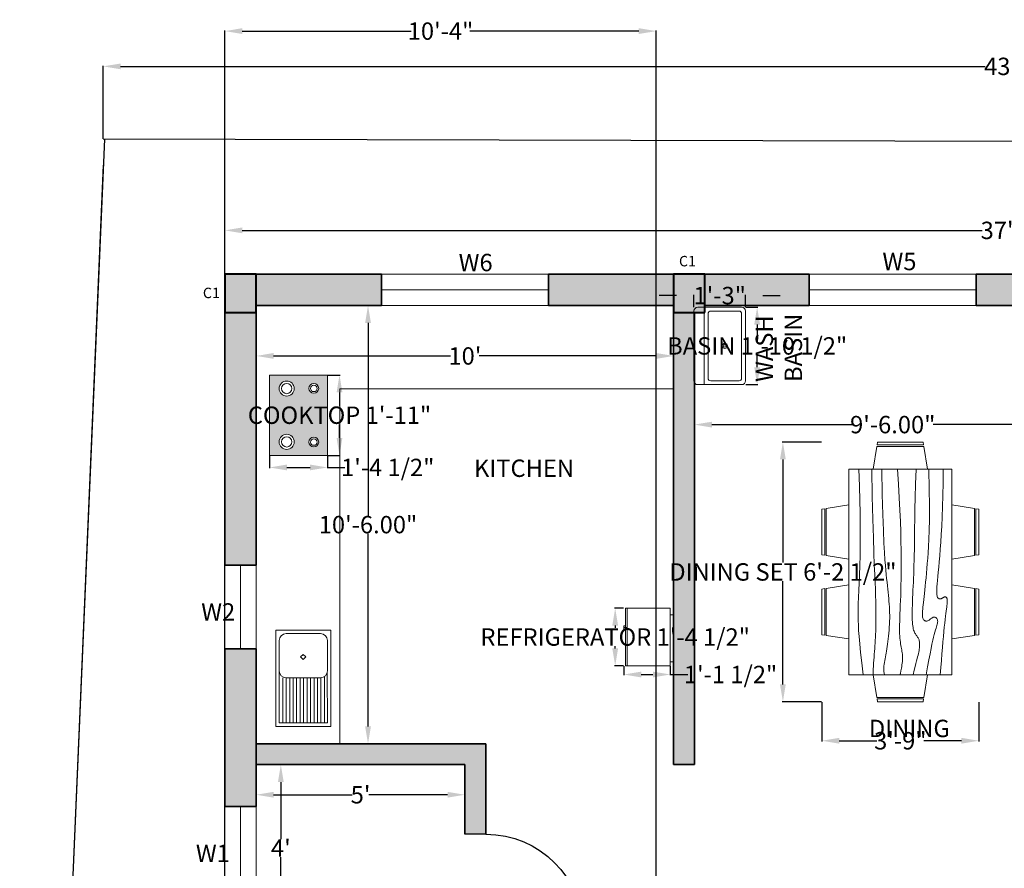
# Model space of a CAD drawing. Units: inches. Extents: x 23868 to 24454, y 31838 to 32477.
# Tile 3 of 4: x 23868 to 24151, y 32233 to 32477. Entities that reach past the tile are written whole.
import ezdxf

# ---------------------------------------------------------------- set-up
doc = ezdxf.new("R2010")
doc.units = ezdxf.units.IN
for name, color, linetype, lineweight in [('A-ANNO-DIMS', 2, 'Continuous', 18), ('A-AREA-IDEN', 7, 'Continuous', 25), ('A-COLS', 7, 'Continuous', 40), ('A-EQPM', 30, 'Continuous', 18), ('A-FIXT-PATT', 30, 'Continuous', 13), ('A-FLOR-CASE', 30, 'Continuous', 18), ('A-FLOR-FIXT', 30, 'Continuous', 18), ('A-FURN', 30, 'Continuous', 18), ('A-GLAZ', 5, 'Continuous', 18), ('A-WALL', 7, 'Continuous', 35), ('C-PROP', 7, 'Continuous', 25), ('door', 1, 'Continuous', 25), ('text', 7, 'Continuous', 18)]:
    doc.layers.add(name, color=color, linetype=linetype, lineweight=lineweight)
doc.layers.add('A-COLS-PATT', color=67, linetype='Continuous', lineweight=13, true_color=0x727430)
doc.layers.add('A-WALL-PATT', color=250, linetype='Continuous', lineweight=13, true_color=0x413a3c)
doc.styles.get("Standard").update_dxf_attribs({"font": 'arial.ttf', "height": 5})
doc.styles.add('style1', font='arial.ttf', dxfattribs={"height": 3})
doc.dimstyles.get("Standard").update_dxf_attribs({"dimtxt": 5, "dimasz": 5, "dimexe": 0.18, "dimexo": 0.0625, "dimgap": 0.09, "dimtad": 0, "dimtih": 1, "dimtoh": 1, "dimzin": 0, "dimdsep": 46, "dimlunit": 3, "dimtxsty": 'Standard', "dimcen": 0.09, "dimadec": 0, "dimazin": 0, "dimtfac": 1, "dimtofl": 0, "dimtmove": 0, "dimatfit": 3, "dimfxl": 1, "dimtolj": 1, "dimtzin": 0, "dimarcsym": 0})

# ---------------------------------------------------------------- blocks, each defined once
blk = doc.blocks.new('*U5')
for p, q in [((0, 0), (0, -6)), ((28, 0), (28, -6))]:
    blk.add_line(p, q)
blk.add_lwpolyline([(0, 0), (0, 28), (1.75, 28), (1.75, 0)], close=True)
blk.add_arc((0, 0), 28, 0, 90)
blk = doc.blocks.new('stov')
h = blk.add_hatch(color=256)
h.dxf.hatch_style = 1
h.set_gradient(color1=(255, 255, 255), color2=(147, 149, 152), name='CYLINDER')
h.paths.add_polyline_path([(0, 0), (16.67, 0), (16.67, 23.1), (0, 23.1)])
h.paths.add_polyline_path([(2.78, 19.21, -1), (7.12, 19.21, -1)], flags=16)
h.paths.add_polyline_path([(3.47, 19.21, -1), (6.43, 19.21, -1)], flags=0)
h.paths.add_polyline_path([(7.12, 3.89, -1), (2.78, 3.89, -1)], flags=16)
h.paths.add_polyline_path([(6.43, 3.89, -1), (3.47, 3.89, -1)], flags=0)
h.paths.add_polyline_path([(11.35, 19.27, -1), (14.15, 19.27, -1)], flags=16)
h.paths.add_polyline_path([(11.81, 19.27, -1), (13.68, 19.27, -1)], flags=0)
h.paths.add_polyline_path([(14.15, 3.83, -1), (11.35, 3.83, -1)], flags=16)
blk.add_lwpolyline([(16.67, 0), (0, 0), (0, 23.1), (16.67, 23.1)], close=True)
for centre, radius in [((4.95, 19.21), 2.17), ((4.95, 19.21), 2.17), ((4.95, 19.21), 1.48), ((12.75, 19.27), 1.4), ((12.75, 19.27), 0.936), ((4.95, 3.89), 2.17), ((4.95, 3.89), 2.17), ((4.95, 3.89), 1.48), ((12.75, 3.83), 1.4), ((12.75, 3.83), 0.936)]:
    blk.add_circle(centre, radius)
blk = doc.blocks.new('Refrigerator-2 door - 36 in top')
for p, q in [((0, -26.999999), (36, -26.999999)), ((11, -27.999999), (11, -28.999999)), ((11, -28.999999), (13, -28.999999)), ((12, -26.999999), (12, -28.999999)), ((13, -28.999999), (13, -27.999999))]:
    blk.add_line(p, q)
blk.add_lwpolyline([(0, -27.999999), (0, 0), (36, 0), (36, -27.999999)], close=True)
blk = doc.blocks.new('Sink-single - 30 in top')
blk.add_line((-15, -3.999996), (15, -3.999996))
for points in [[(-13.5, 0), (13.5, 0)], [(-15, -18.499996), (-15, -1.5)], [(15, -1.5), (15, -18.499996)], [(-13.5, -17.499996), (-13.5, -6.499996)], [(-12.5, -5.499996), (12.5, -5.499996)], [(13.5, -6.499996), (13.5, -17.499996)], [(12.5, -18.499996), (-12.5, -18.499996)], [(13.5, -19.999996), (-13.5, -19.999996)]]:
    blk.add_lwpolyline(points)
for radius in [1, 0.5]:
    blk.add_circle((0, -11.999996), radius)
for centre, radius, start, end in [((-13.5, -1.5), 1.5, 90, 180), ((13.5, -1.5), 1.5, 0, 90), ((-12.5, -6.499996), 1, 90, 180), ((12.5, -6.499996), 1, 0, 90), ((-13.5, -18.499996), 1.5, 180, 270), ((-12.5, -17.499996), 1, 180, 270), ((12.5, -17.499996), 1, 270, 0), ((13.5, -18.499996), 1.5, 270, 0)]:
    blk.add_arc(centre, radius, start, end)
blk = doc.blocks.new('Dining Set - 36 x 72 in.')
for p, q in [((-22.2343, 26.00059), (-23.4847, 17.99762)), ((-22.2304, 26), (-5.7608, 26)), ((-22, 27.5), (-22.1562, 26.50042)), ((-5.8416, 26.5), (-22.1534, 26.5)), ((-22, 27.5), (-6, 27.5)), ((-5.8437, 26.49966), (-6, 27.5)), ((-4.5152, 17.99762), (-5.7655, 25.99926)), ((5.7657, 26.00059), (4.5153, 17.99762)), ((5.7696, 26), (22.2392, 26)), ((6, 27.5), (5.8438, 26.50042)), ((22.1584, 26.5), (5.8466, 26.5)), ((6, 27.5), (22, 27.5)), ((22.1563, 26.49966), (22, 27.5)), ((23.4848, 17.99762), (22.2345, 25.99926)), ((36, 18), (-36, 18)), ((-36, 18), (-36, -18)), ((36, -18), (36, 18)), ((-45.5, 8), (-44.5004, 8.15617)), ((-45.5, 8), (-45.5, -8)), ((-44.5, -8.15843), (-44.5, 8.15338)), ((-44.0006, 8.23428), (-35.9976, 9.48474)), ((-44, 8.23041), (-44, -8.23915)), ((44.0006, 8.23428), (35.9976, 9.48474)), ((44, 8.23041), (44, -8.23915)), ((44.5, -8.15843), (44.5, 8.15338)), ((45.5, 8), (44.5005, 8.15617)), ((45.5, 8), (45.5, -8)), ((-44.4997, -8.15631), (-45.5, -8)), ((-35.9976, -9.48476), (-43.9993, -8.2345)), ((35.9976, -9.48476), (43.9993, -8.2345)), ((44.4997, -8.15631), (45.5, -8)), ((-36, -18), (36, -18)), ((-22.2343, -26.0006), (-23.4847, -17.99762)), ((-4.5152, -17.99762), (-5.7655, -25.99928)), ((5.7657, -26.0006), (4.5153, -17.99762)), ((23.4848, -17.99762), (22.2345, -25.99928)), ((-22.2304, -26), (-5.7608, -26)), ((-22, -27.5), (-22.1562, -26.50044)), ((-5.8416, -26.5), (-22.1534, -26.5)), ((-22, -27.5), (-6, -27.5)), ((-5.8437, -26.49967), (-6, -27.5)), ((5.7696, -26), (22.2392, -26)), ((6, -27.5), (5.8438, -26.50044)), ((22.1584, -26.5), (5.8466, -26.5)), ((6, -27.5), (22, -27.5)), ((22.1563, -26.49967), (22, -27.5))]:
    blk.add_line(p, q)
for points in [[(-36, 15), (-31.1772, 14.97754), (-26.8079, 14.91406), (-22.8538, 14.81543), (-19.276, 14.6875), (-16.0362, 14.53613), (-13.0957, 14.36718), (-10.4159, 14.18652), (-7.9583, 14), (-5.6904, 13.81315), (-3.6035, 13.63021), (-1.6954, 13.45508), (0.0365, 13.29166), (1.5945, 13.14388), (2.9811, 13.01562), (4.1988, 12.9108), (5.25, 12.83333), (6.1393, 12.78613), (6.8802, 12.76823), (7.4883, 12.77767), (7.9792, 12.8125), (8.3685, 12.87077), (8.6719, 12.95052), (8.9049, 13.0498), (9.0833, 13.16666), (9.2205, 13.29899), (9.3216, 13.44401), (9.3895, 13.59879), (9.4271, 13.76041), (9.4373, 13.92594), (9.4232, 14.09245), (9.3875, 14.257), (9.3333, 14.41666), (9.2638, 14.56917), (9.1836, 14.71484), (9.0975, 14.85465), (9.0104, 14.98958), (8.9272, 15.1206), (8.8529, 15.2487), (8.7922, 15.37483), (8.75, 15.5), (8.7305, 15.62467), (8.7344, 15.74739), (8.7617, 15.86621), (8.8125, 15.97916), (8.8867, 16.08431), (8.9844, 16.17968), (9.1055, 16.26334), (9.25, 16.33333), (9.4189, 16.38802), (9.6172, 16.42708), (9.8506, 16.45052), (10.125, 16.45833), (10.4463, 16.45052), (10.8203, 16.42708), (11.2529, 16.38802), (11.75, 16.33333), (12.3184, 16.26318), (12.9694, 16.17838), (13.7151, 16.07991), (14.5677, 15.96875), (15.5395, 15.84586), (16.6426, 15.71224), (17.8893, 15.56884), (19.2917, 15.41666), (20.859, 15.25667), (22.5879, 15.08984), (24.4721, 14.91715), (26.5052, 14.73958), (28.6809, 14.5581), (30.9929, 14.3737), (33.4347, 14.18733), (36, 14)], [(-36, 10), (-28.9766, 10.14274), (-23.1725, 10.20442), (-18.4241, 10.19775), (-14.5677, 10.13541), (-11.4399, 10.03011), (-8.877, 9.89453), (-6.7154, 9.74137), (-4.7917, 9.58333), (-2.9698, 9.43082), (-1.2246, 9.28515), (0.4415, 9.14534), (2.026, 9.01041), (3.5266, 8.87939), (4.9408, 8.7513), (6.266, 8.62516), (7.5, 8.5), (8.6411, 8.37549), (9.6914, 8.2539), (10.6538, 8.13818), (11.5312, 8.03125), (12.3267, 7.93603), (13.043, 7.85547), (13.6831, 7.79248), (14.25, 7.75), (14.7471, 7.7303), (15.1797, 7.73307), (15.5537, 7.75732), (15.875, 7.80208), (16.1494, 7.86637), (16.3828, 7.94922), (16.5811, 8.04964), (16.75, 8.16666), (16.8944, 8.29915), (17.0143, 8.44531), (17.1089, 8.60319), (17.1771, 8.77083), (17.218, 8.94629), (17.2305, 9.1276), (17.2137, 9.31282), (17.1667, 9.5), (17.0895, 9.6875), (16.987, 9.875), (16.8649, 10.0625), (16.7292, 10.25), (16.5856, 10.4375), (16.4401, 10.625), (16.2985, 10.8125), (16.1667, 11), (16.05, 11.18733), (15.9518, 11.3737), (15.8752, 11.5581), (15.8229, 11.73958), (15.798, 11.91715), (15.8034, 12.08984), (15.842, 12.25667), (15.9167, 12.41666), (16.0295, 12.56836), (16.1784, 12.70833), (16.3605, 12.83268), (16.5729, 12.9375), (16.8127, 13.01888), (17.0768, 13.07291), (17.3625, 13.0957), (17.6667, 13.08333), (17.9894, 13.03312), (18.3418, 12.94726), (18.7382, 12.82918), (19.1927, 12.68229), (19.7195, 12.51001), (20.3327, 12.31575), (21.0465, 12.10294), (21.875, 11.875), (22.8357, 11.63354), (23.959, 11.37304), (25.2786, 11.08618), (26.8282, 10.76562), (28.6414, 10.40405), (30.752, 9.99414), (33.1936, 9.52856), (36, 9)], [(-36, 5.5), (-30.7157, 5.3348), (-26.069, 5.20963), (-21.9946, 5.11767), (-18.4271, 5.05208), (-15.3009, 5.00602), (-12.5508, 4.97265), (-10.1112, 4.94515), (-7.9167, 4.91666), (-5.909, 4.88167), (-4.0586, 4.83984), (-2.3429, 4.79215), (-0.7396, 4.73958), (0.7739, 4.6831), (2.22, 4.6237), (3.6213, 4.56233), (5, 4.5), (6.373, 4.43782), (7.7344, 4.3776), (9.0723, 4.32129), (10.375, 4.27083), (11.6309, 4.22819), (12.8281, 4.19531), (13.9551, 4.17415), (15, 4.16666), (15.954, 4.17448), (16.819, 4.19791), (17.6001, 4.23698), (18.3021, 4.29166), (18.9299, 4.36198), (19.4883, 4.44791), (19.9823, 4.54948), (20.4167, 4.66666), (20.7969, 4.79899), (21.1302, 4.94401), (21.4245, 5.09879), (21.6875, 5.26041), (21.9271, 5.42594), (22.1511, 5.59245), (22.3672, 5.757), (22.5834, 5.91666), (22.8065, 6.06868), (23.0404, 6.21093), (23.2879, 6.34147), (23.5521, 6.45833), (23.8358, 6.55957), (24.142, 6.64323), (24.4735, 6.70735), (24.8334, 6.75), (25.2235, 6.76969), (25.642, 6.76692), (26.0858, 6.74267), (26.5521, 6.69791), (27.0379, 6.63362), (27.5404, 6.55078), (28.0565, 6.45036), (28.5834, 6.33333), (29.1242, 6.19987), (29.7071, 6.04687), (30.3661, 5.87044), (31.1354, 5.66666), (32.0493, 5.43164), (33.142, 5.16146), (34.4475, 4.85221), (36, 4.5)], [(-36, -1), (-30.7915, -0.6591), (-26.0195, -0.38216), (-21.6519, -0.16284), (-17.6563, 0.00521), (-14.0005, 0.12833), (-10.6523, 0.21289), (-7.5796, 0.26522), (-4.75, 0.29166), (-2.134, 0.29793), (0.2878, 0.28711), (2.5317, 0.26163), (4.6146, 0.22396), (6.5529, 0.17651), (8.3633, 0.12174), (10.0623, 0.06209), (11.6667, 0), (13.1899, -0.06201), (14.6341, -0.1211), (15.9982, -0.17432), (17.2813, -0.21875), (18.4823, -0.25147), (19.6003, -0.26953), (20.6343, -0.27002), (21.5834, -0.25), (22.4481, -0.20768), (23.2357, -0.14584), (23.9549, -0.06836), (24.6146, 0.02083), (25.2235, 0.11784), (25.7904, 0.21875), (26.3241, 0.31966), (26.8334, 0.41666), (27.3265, 0.50618), (27.8099, 0.58593), (28.2894, 0.65397), (28.7709, 0.70833), (29.2601, 0.74707), (29.763, 0.76823), (30.2855, 0.76985), (30.8334, 0.75), (31.4088, 0.70784), (31.9994, 0.64713), (32.589, 0.57275), (33.1615, 0.48958), (33.7008, 0.4025), (34.1908, 0.3164), (34.6153, 0.23616), (34.9584, 0.16666), (35.2099, 0.11165), (35.3848, 0.07031), (35.504, 0.04069), (35.5886, 0.02083), (35.6594, 0.00879), (35.7377, 0.0026), (35.8442, 0.00032), (36, 0)], [(-36, -6.5), (-27.1843, -6.31267), (-20.084, -6.1263), (-14.469, -5.9419), (-10.1094, -5.76042), (-6.7752, -5.58285), (-4.2363, -5.41016), (-2.2629, -5.24333), (-0.625, -5.08334), (0.8708, -4.93099), (2.2715, -4.78646), (3.5872, -4.64974), (4.8281, -4.52084), (6.0046, -4.39974), (7.127, -4.28646), (8.2053, -4.18099), (9.25, -4.08334), (10.2705, -3.99382), (11.2734, -3.91407), (12.2647, -3.84603), (13.25, -3.79167), (14.2354, -3.75293), (15.2266, -3.73177), (16.2295, -3.73015), (17.25, -3.75), (18.2912, -3.79248), (19.3451, -3.85547), (20.4009, -3.93604), (21.4479, -4.03125), (22.4754, -4.13819), (23.4727, -4.25391), (24.4289, -4.37549), (25.3334, -4.5), (26.1785, -4.62492), (26.9694, -4.74935), (27.7145, -4.87281), (28.4219, -4.99479), (29.1, -5.11483), (29.7572, -5.23242), (30.4016, -5.34709), (31.0417, -5.45834), (31.6837, -5.56437), (32.3262, -5.65821), (32.9658, -5.73153), (33.599, -5.77604), (34.2224, -5.78345), (34.8327, -5.74545), (35.4264, -5.65373), (36, -5.5)], [(-36, -10), (-26.4022, -9.81299), (-18.4675, -9.62891), (-11.9839, -9.45069), (-6.7396, -9.28125), (-2.5226, -9.12354), (0.8789, -8.98047), (3.6769, -8.85498), (6.0833, -8.75), (8.2767, -8.66765), (10.3021, -8.60677), (12.1712, -8.56543), (13.8958, -8.54167), (15.4876, -8.53353), (16.9583, -8.53907), (18.3197, -8.55632), (19.5834, -8.58334), (20.7616, -8.61841), (21.8685, -8.66081), (22.9188, -8.71004), (23.9271, -8.76563), (24.9081, -8.82707), (25.8763, -8.89388), (26.8465, -8.96558), (27.8334, -9.04167), (28.8474, -9.12118), (29.8828, -9.20117), (30.93, -9.27824), (31.9792, -9.34896), (33.0205, -9.40991), (34.0443, -9.45768), (35.0407, -9.48885), (36, -9.5)], [(-36, -14.5), (-30.0881, -14.33513), (-25.0332, -14.21224), (-20.7312, -14.12647), (-17.0781, -14.07292), (-13.97, -14.04671), (-11.3027, -14.04297), (-8.9724, -14.05681), (-6.875, -14.08334), (-4.9224, -14.11833), (-3.0905, -14.16016), (-1.3709, -14.20785), (0.2448, -14.26042), (1.7647, -14.3169), (3.1973, -14.3763), (4.5507, -14.43767), (5.8333, -14.5), (7.0554, -14.5621), (8.235, -14.62175), (9.3922, -14.67652), (10.5469, -14.72396), (11.7192, -14.76164), (12.929, -14.78711), (14.1965, -14.79794), (15.5417, -14.79167), (16.9933, -14.76424), (18.6152, -14.70508), (20.4804, -14.60197), (22.6615, -14.44271), (25.2312, -14.21509), (28.2624, -13.9069), (31.8277, -13.50594), (36, -13)]]:
    blk.add_lwpolyline(points)
blk = doc.blocks.new('*D17')
at = {"layer": 'A-ANNO-DIMS', "color": 0, "lineweight": -2, "transparency": 16777216}
for p, q in [((23969.04, 32394.61), (23968.06, 32394.61)), ((23968.24, 32389.61), (23968.24, 32334.25)), ((23968.24, 32273.61), (23968.24, 32328.97)), ((23969.04, 32268.61), (23968.06, 32268.61))]:
    blk.add_line(p, q, dxfattribs=at)
at = {"layer": 'A-ANNO-DIMS', "color": 0, "transparency": 16777216}
for points in [[(23967.41, 32389.61), (23969.08, 32389.61), (23968.24, 32394.61)], [(23967.41, 32273.61), (23969.08, 32273.61), (23968.24, 32268.61)]]:
    blk.add_solid(points, dxfattribs=at)
at = {"layer": 'Defpoints', "color": 0, "transparency": 16777216}
for p in [(23968.24, 32394.61), (23969.1, 32394.61), (23969.1, 32268.61)]:
    blk.add_point(p, dxfattribs=at)
at = {"layer": 'A-ANNO-DIMS', "color": 0, "transparency": 16777216, "insert": (23968.24, 32331.61), "char_height": 5, "attachment_point": 5}
blk.add_mtext('\\A1;10\'-6.00"', dxfattribs=at)
blk = doc.blocks.new('*D18')
at = {"layer": 'A-ANNO-DIMS', "color": 0, "lineweight": -2, "transparency": 16777216}
for p, q in [((23936.1, 32387.07), (23936.1, 32379.93)), ((24056.1, 32387.07), (24056.1, 32379.93)), ((23941.1, 32380.11), (23992, 32380.11)), ((24051.1, 32380.11), (24000.2, 32380.11))]:
    blk.add_line(p, q, dxfattribs=at)
at = {"layer": 'A-ANNO-DIMS', "color": 0, "transparency": 16777216}
for points in [[(23941.1, 32380.95), (23941.1, 32379.28), (23936.1, 32380.11)], [(24051.1, 32380.95), (24051.1, 32379.28), (24056.1, 32380.11)]]:
    blk.add_solid(points, dxfattribs=at)
at = {"layer": 'Defpoints', "color": 0, "transparency": 16777216}
for p in [(23936.1, 32387.13), (24056.1, 32387.13), (23936.1, 32380.11)]:
    blk.add_point(p, dxfattribs=at)
at = {"layer": 'A-ANNO-DIMS', "color": 0, "transparency": 16777216, "insert": (23996.1, 32380.11), "char_height": 5, "attachment_point": 5}
blk.add_mtext("\\A1;10'", dxfattribs=at)
blk = doc.blocks.new('*D19')
at = {"layer": 'A-ANNO-DIMS', "color": 0, "lineweight": -2, "transparency": 16777216}
for p, q in [((24062.1, 32354.55), (24062.1, 32360.55)), ((24067.1, 32360.37), (24107.51, 32360.37)), ((24171.1, 32360.37), (24130.69, 32360.37)), ((24176.1, 32354.55), (24176.1, 32360.55))]:
    blk.add_line(p, q, dxfattribs=at)
at = {"layer": 'A-ANNO-DIMS', "color": 0, "transparency": 16777216}
for points in [[(24067.1, 32361.2), (24067.1, 32359.53), (24062.1, 32360.37)], [(24171.1, 32361.2), (24171.1, 32359.53), (24176.1, 32360.37)]]:
    blk.add_solid(points, dxfattribs=at)
at = {"layer": 'Defpoints', "color": 0, "transparency": 16777216}
for p in [(24062.1, 32360.37), (24062.1, 32354.49), (24176.1, 32354.49)]:
    blk.add_point(p, dxfattribs=at)
at = {"layer": 'A-ANNO-DIMS', "color": 0, "transparency": 16777216, "insert": (24119.1, 32360.37), "char_height": 5, "attachment_point": 5}
blk.add_mtext('\\A1;9\'-6.00"', dxfattribs=at)
blk = doc.blocks.new('*D32')
at = {"layer": 'A-ANNO-DIMS', "color": 0, "lineweight": -2, "transparency": 16777216}
for p, q in [((23927.1, 32403.67), (23927.1, 32416.39)), ((23932.1, 32416.21), (24144.77, 32416.21)), ((24366.1, 32416.21), (24153.43, 32416.21)), ((24371.1, 32403.67), (24371.1, 32416.39))]:
    blk.add_line(p, q, dxfattribs=at)
at = {"layer": 'A-ANNO-DIMS', "color": 0, "transparency": 16777216}
for points in [[(23932.1, 32417.05), (23932.1, 32415.38), (23927.1, 32416.21)], [(24366.1, 32417.05), (24366.1, 32415.38), (24371.1, 32416.21)]]:
    blk.add_solid(points, dxfattribs=at)
at = {"layer": 'Defpoints', "color": 0, "transparency": 16777216}
for p in [(24371.1, 32416.21), (23927.1, 32403.61), (24371.1, 32403.61)]:
    blk.add_point(p, dxfattribs=at)
at = {"layer": 'A-ANNO-DIMS', "color": 0, "transparency": 16777216, "insert": (24149.1, 32416.21), "char_height": 5, "attachment_point": 5}
blk.add_mtext("\\A1;37'", dxfattribs=at)
blk = doc.blocks.new('*D35')
at = {"layer": 'A-ANNO-DIMS', "color": 0, "lineweight": -2, "transparency": 16777216}
for p, q in [((23936.16, 32262.61), (23943.36, 32262.61)), ((23943.18, 32257.61), (23943.18, 32241.2)), ((23943.18, 32219.61), (23943.18, 32236.02)), ((23936.16, 32214.61), (23943.36, 32214.61))]:
    blk.add_line(p, q, dxfattribs=at)
at = {"layer": 'A-ANNO-DIMS', "color": 0, "transparency": 16777216}
for points in [[(23942.35, 32257.61), (23944.01, 32257.61), (23943.18, 32262.61)], [(23942.35, 32219.61), (23944.01, 32219.61), (23943.18, 32214.61)]]:
    blk.add_solid(points, dxfattribs=at)
at = {"layer": 'Defpoints', "color": 0, "transparency": 16777216}
for p in [(23936.1, 32262.61), (23943.18, 32262.61), (23936.1, 32214.61)]:
    blk.add_point(p, dxfattribs=at)
at = {"layer": 'A-ANNO-DIMS', "color": 0, "transparency": 16777216, "insert": (23943.18, 32238.61), "char_height": 5, "attachment_point": 5}
blk.add_mtext("\\A1;4'", dxfattribs=at)
blk = doc.blocks.new('*D36')
at = {"layer": 'A-ANNO-DIMS', "color": 0, "lineweight": -2, "transparency": 16777216}
for p, q in [((23936.1, 32256.55), (23936.1, 32253.77)), ((23996.1, 32256.55), (23996.1, 32253.77)), ((23941.1, 32253.95), (23963.71, 32253.95)), ((23991.1, 32253.95), (23968.49, 32253.95))]:
    blk.add_line(p, q, dxfattribs=at)
at = {"layer": 'A-ANNO-DIMS', "color": 0, "transparency": 16777216}
for points in [[(23941.1, 32254.79), (23941.1, 32253.12), (23936.1, 32253.95)], [(23991.1, 32254.79), (23991.1, 32253.12), (23996.1, 32253.95)]]:
    blk.add_solid(points, dxfattribs=at)
at = {"layer": 'Defpoints', "color": 0, "transparency": 16777216}
for p in [(23936.1, 32256.61), (23996.1, 32256.61), (23996.1, 32253.95)]:
    blk.add_point(p, dxfattribs=at)
at = {"layer": 'A-ANNO-DIMS', "color": 0, "transparency": 16777216, "insert": (23966.1, 32253.95), "char_height": 5, "attachment_point": 5}
blk.add_mtext("\\A1;5'", dxfattribs=at)
blk = doc.blocks.new('*D42')
at = {"layer": 'A-ANNO-DIMS', "color": 0, "lineweight": -2, "transparency": 16777216}
for p, q in [((23892.1, 32442.52), (23892.1, 32463.54)), ((23897.1, 32463.36), (24145.67, 32463.36)), ((24403.1, 32463.36), (24154.53, 32463.36)), ((24408.1, 32441.11), (24408.1, 32463.54))]:
    blk.add_line(p, q, dxfattribs=at)
at = {"layer": 'A-ANNO-DIMS', "color": 0, "transparency": 16777216}
for points in [[(23897.1, 32464.19), (23897.1, 32462.53), (23892.1, 32463.36)], [(24403.1, 32464.19), (24403.1, 32462.53), (24408.1, 32463.36)]]:
    blk.add_solid(points, dxfattribs=at)
at = {"layer": 'Defpoints', "color": 0, "transparency": 16777216}
for p in [(23892.1, 32463.36), (23892.1, 32442.45), (24408.1, 32441.05)]:
    blk.add_point(p, dxfattribs=at)
at = {"layer": 'A-ANNO-DIMS', "color": 0, "transparency": 16777216, "insert": (24150.1, 32463.36), "char_height": 5, "attachment_point": 5}
blk.add_mtext("\\A1;43'", dxfattribs=at)
blk = doc.blocks.new('WIN-48IN')
blk.add_line((0, 4.5), (48, 4.5))
blk.add_lwpolyline([(0, 0), (48, 0), (48, 9), (0, 9)], close=True)
blk = doc.blocks.new('WIN-24IN')
blk.add_line((4.5, 0), (4.5, 24))
blk.add_lwpolyline([(0, 24), (9, 24), (9, 0), (0, 0)], close=True)
blk = doc.blocks.new('COL-C1')
blk.add_lwpolyline([(9, 0), (9, 11.01), (0, 11.01), (0, 0)], close=True)
blk = doc.blocks.new('*D59')
at = {"layer": 'A-ANNO-DIMS', "color": 0, "lineweight": -2, "transparency": 16777216}
for p, q in [((23956.64, 32374.62), (23960.22, 32374.62)), ((23960.04, 32369.62), (23960.04, 32365.74)), ((23960.04, 32356.52), (23960.04, 32360.39)), ((23956.64, 32351.52), (23960.22, 32351.52))]:
    blk.add_line(p, q, dxfattribs=at)
at = {"layer": 'A-ANNO-DIMS', "color": 0, "transparency": 16777216}
for points in [[(23959.21, 32369.62), (23960.88, 32369.62), (23960.04, 32374.62)], [(23959.21, 32356.52), (23960.88, 32356.52), (23960.04, 32351.52)]]:
    blk.add_solid(points, dxfattribs=at)
at = {"layer": 'Defpoints', "color": 0, "transparency": 16777216}
for p in [(23956.58, 32374.62), (23960.04, 32374.62), (23956.58, 32351.52)]:
    blk.add_point(p, dxfattribs=at)
at = {"layer": 'A-ANNO-DIMS', "color": 0, "transparency": 16777216, "insert": (23960.04, 32363.07), "char_height": 5, "attachment_point": 5}
blk.add_mtext('\\A1;COOKTOP 1\'-11"', dxfattribs=at)
blk = doc.blocks.new('*D60')
at = {"layer": 'A-ANNO-DIMS', "color": 0, "lineweight": -2, "transparency": 16777216}
for p, q in [((23939.91, 32351.45), (23939.91, 32347.87)), ((23956.58, 32351.45), (23956.58, 32347.87)), ((23944.91, 32348.05), (23951.58, 32348.05)), ((23956.58, 32348.05), (23961.58, 32348.05))]:
    blk.add_line(p, q, dxfattribs=at)
at = {"layer": 'A-ANNO-DIMS', "color": 0, "transparency": 16777216}
for points in [[(23944.91, 32348.88), (23944.91, 32347.22), (23939.91, 32348.05)], [(23951.58, 32348.88), (23951.58, 32347.22), (23956.58, 32348.05)]]:
    blk.add_solid(points, dxfattribs=at)
at = {"layer": 'Defpoints', "color": 0, "transparency": 16777216}
for p in [(23939.91, 32351.52), (23956.58, 32351.52), (23956.58, 32348.05)]:
    blk.add_point(p, dxfattribs=at)
at = {"layer": 'A-ANNO-DIMS', "color": 0, "transparency": 16777216, "insert": (23973.91, 32348.05), "char_height": 5, "attachment_point": 5}
blk.add_mtext('\\A1;1\'-4 1/2"', dxfattribs=at)
blk = doc.blocks.new('*D61')
at = {"layer": 'A-ANNO-DIMS', "color": 0, "lineweight": -2, "transparency": 16777216}
for p, q in [((24041.72, 32307.6), (24039.12, 32307.6)), ((24039.3, 32302.6), (24039.3, 32301.98)), ((24039.3, 32296.01), (24039.3, 32296.63)), ((24041.72, 32291.01), (24039.12, 32291.01))]:
    blk.add_line(p, q, dxfattribs=at)
at = {"layer": 'A-ANNO-DIMS', "color": 0, "transparency": 16777216}
for points in [[(24038.47, 32302.6), (24040.13, 32302.6), (24039.3, 32307.6)], [(24038.47, 32296.01), (24040.13, 32296.01), (24039.3, 32291.01)]]:
    blk.add_solid(points, dxfattribs=at)
at = {"layer": 'Defpoints', "color": 0, "transparency": 16777216}
for p in [(24041.79, 32307.6), (24039.3, 32291.01), (24041.79, 32291.01)]:
    blk.add_point(p, dxfattribs=at)
at = {"layer": 'A-ANNO-DIMS', "color": 0, "transparency": 16777216, "insert": (24039.3, 32299.3), "char_height": 5, "attachment_point": 5}
blk.add_mtext('\\A1;REFRIGERATOR 1\'-4 1/2"', dxfattribs=at)
blk = doc.blocks.new('*D62')
at = {"layer": 'A-ANNO-DIMS', "color": 0, "lineweight": -2, "transparency": 16777216}
for p, q in [((24041.79, 32290.95), (24041.79, 32288.34)), ((24055.15, 32290.95), (24055.15, 32288.34)), ((24046.79, 32288.52), (24050.15, 32288.52)), ((24055.15, 32288.52), (24060.15, 32288.52))]:
    blk.add_line(p, q, dxfattribs=at)
at = {"layer": 'A-ANNO-DIMS', "color": 0, "transparency": 16777216}
for points in [[(24046.79, 32289.35), (24046.79, 32287.69), (24041.79, 32288.52)], [(24050.15, 32289.35), (24050.15, 32287.69), (24055.15, 32288.52)]]:
    blk.add_solid(points, dxfattribs=at)
at = {"layer": 'Defpoints', "color": 0, "transparency": 16777216}
for p in [(24041.79, 32291.01), (24055.15, 32291.01), (24055.15, 32288.52)]:
    blk.add_point(p, dxfattribs=at)
at = {"layer": 'A-ANNO-DIMS', "color": 0, "transparency": 16777216, "insert": (24072.47, 32288.52), "char_height": 5, "attachment_point": 5}
blk.add_mtext('\\A1;1\'-1 1/2"', dxfattribs=at)
blk = doc.blocks.new('*D63')
at = {"layer": 'A-ANNO-DIMS', "color": 0, "lineweight": -2, "transparency": 16777216}
for p, q in [((24076.84, 32394.12), (24080.3, 32394.12)), ((24080.12, 32389.12), (24080.12, 32385.66)), ((24080.12, 32376.86), (24080.12, 32380.31)), ((24076.84, 32371.86), (24080.3, 32371.86))]:
    blk.add_line(p, q, dxfattribs=at)
at = {"layer": 'A-ANNO-DIMS', "color": 0, "transparency": 16777216}
for points in [[(24079.28, 32389.12), (24080.95, 32389.12), (24080.12, 32394.12)], [(24079.28, 32376.86), (24080.95, 32376.86), (24080.12, 32371.86)]]:
    blk.add_solid(points, dxfattribs=at)
at = {"layer": 'Defpoints', "color": 0, "transparency": 16777216}
for p in [(24076.78, 32394.12), (24080.12, 32394.12), (24076.78, 32371.86)]:
    blk.add_point(p, dxfattribs=at)
at = {"layer": 'A-ANNO-DIMS', "color": 0, "transparency": 16777216, "insert": (24080.12, 32382.99), "char_height": 5, "attachment_point": 5}
blk.add_mtext('\\A1;BASIN 1\'-10 1/2"', dxfattribs=at)
blk = doc.blocks.new('*D64')
at = {"layer": 'A-ANNO-DIMS', "color": 0, "lineweight": -2, "transparency": 16777216}
for p, q in [((24056.94, 32397.46), (24051.94, 32397.46)), ((24061.94, 32394.18), (24061.94, 32397.64)), ((24076.78, 32394.18), (24076.78, 32397.64)), ((24081.78, 32397.46), (24086.78, 32397.46))]:
    blk.add_line(p, q, dxfattribs=at)
at = {"layer": 'A-ANNO-DIMS', "color": 0, "transparency": 16777216}
for points in [[(24056.94, 32398.29), (24056.94, 32396.62), (24061.94, 32397.46)], [(24081.78, 32398.29), (24081.78, 32396.62), (24076.78, 32397.46)]]:
    blk.add_solid(points, dxfattribs=at)
at = {"layer": 'Defpoints', "color": 0, "transparency": 16777216}
for p in [(24061.94, 32397.46), (24061.94, 32394.12), (24076.78, 32394.12)]:
    blk.add_point(p, dxfattribs=at)
at = {"layer": 'A-ANNO-DIMS', "color": 0, "transparency": 16777216, "insert": (24069.36, 32397.46), "char_height": 5, "attachment_point": 5}
blk.add_mtext('\\A1;1\'-3"', dxfattribs=at)
blk = doc.blocks.new('*D65')
at = {"layer": 'A-ANNO-DIMS', "color": 0, "lineweight": -2, "transparency": 16777216}
for p, q in [((24098.65, 32355.34), (24087.34, 32355.34)), ((24087.52, 32350.34), (24087.52, 32320.68)), ((24087.52, 32285.68), (24087.52, 32315.33)), ((24098.65, 32280.68), (24087.34, 32280.68))]:
    blk.add_line(p, q, dxfattribs=at)
at = {"layer": 'A-ANNO-DIMS', "color": 0, "transparency": 16777216}
for points in [[(24086.68, 32350.34), (24088.35, 32350.34), (24087.52, 32355.34)], [(24086.68, 32285.68), (24088.35, 32285.68), (24087.52, 32280.68)]]:
    blk.add_solid(points, dxfattribs=at)
at = {"layer": 'Defpoints', "color": 0, "transparency": 16777216}
for p in [(24098.72, 32355.34), (24087.52, 32280.68), (24098.72, 32280.68)]:
    blk.add_point(p, dxfattribs=at)
at = {"layer": 'A-ANNO-DIMS', "color": 0, "transparency": 16777216, "insert": (24087.52, 32318.01), "char_height": 5, "attachment_point": 5}
blk.add_mtext('\\A1;DINING SET 6\'-2 1/2"', dxfattribs=at)
blk = doc.blocks.new('*D66')
at = {"layer": 'A-ANNO-DIMS', "color": 0, "lineweight": -2, "transparency": 16777216}
for p, q in [((24098.72, 32280.61), (24098.72, 32269.3)), ((24143.84, 32280.61), (24143.84, 32269.3)), ((24103.72, 32269.48), (24114.54, 32269.48)), ((24138.84, 32269.48), (24128.01, 32269.48))]:
    blk.add_line(p, q, dxfattribs=at)
at = {"layer": 'A-ANNO-DIMS', "color": 0, "transparency": 16777216}
for points in [[(24103.72, 32270.31), (24103.72, 32268.64), (24098.72, 32269.48)], [(24138.84, 32270.31), (24138.84, 32268.64), (24143.84, 32269.48)]]:
    blk.add_solid(points, dxfattribs=at)
at = {"layer": 'Defpoints', "color": 0, "transparency": 16777216}
for p in [(24098.72, 32280.68), (24143.84, 32280.68), (24143.84, 32269.48)]:
    blk.add_point(p, dxfattribs=at)
at = {"layer": 'A-ANNO-DIMS', "color": 0, "transparency": 16777216, "insert": (24121.28, 32269.48), "char_height": 5, "attachment_point": 5}
blk.add_mtext('\\A1;3\'-9"', dxfattribs=at)
blk = doc.blocks.new('*D70')
at = {"layer": 'A-ANNO-DIMS', "color": 0, "lineweight": -2, "transparency": 16777216}
for p, q in [((23927.1, 32214.67), (23927.1, 32473.68)), ((23932.1, 32473.5), (23980.65, 32473.5)), ((24046.09, 32473.5), (23997.54, 32473.5)), ((24051.09, 32216.17), (24051.09, 32473.68))]:
    blk.add_line(p, q, dxfattribs=at)
at = {"layer": 'A-ANNO-DIMS', "color": 0, "transparency": 16777216}
for points in [[(23932.1, 32474.34), (23932.1, 32472.67), (23927.1, 32473.5)], [(24046.09, 32474.34), (24046.09, 32472.67), (24051.09, 32473.5)]]:
    blk.add_solid(points, dxfattribs=at)
at = {"layer": 'Defpoints', "color": 0, "transparency": 16777216}
for p in [(24051.09, 32473.5), (23927.1, 32214.61), (24051.09, 32216.11)]:
    blk.add_point(p, dxfattribs=at)
at = {"layer": 'A-ANNO-DIMS', "color": 0, "transparency": 16777216, "insert": (23989.09, 32473.5), "char_height": 5, "attachment_point": 5}
blk.add_mtext('\\A1;10\'-4"', dxfattribs=at)

msp = doc.modelspace()

# ---------------------------------------------------------------- hatches: boundary and pattern name
at = {"layer": 'A-COLS-PATT'}
h = msp.add_hatch(color=256, dxfattribs=at)
h.dxf.hatch_style = 1
h.paths.add_polyline_path([(23938.111, 32028.608), (23927.1, 32028.608), (23927.1, 32019.608), (23938.111, 32019.608)])
h.paths.add_polyline_path([(24049.921, 32028.608), (24038.91, 32028.608), (24038.91, 32019.608), (24049.921, 32019.608)])
h.paths.add_polyline_path([(24184.484, 32028.608), (24173.473, 32028.608), (24173.473, 32019.608), (24184.484, 32019.608)])
h.paths.add_polyline_path([(24371.1, 32028.608), (24360.089, 32028.608), (24360.089, 32019.608), (24371.1, 32019.608)])
h.paths.add_polyline_path([(24371.1, 32214.608), (24362.1, 32214.608), (24362.1, 32203.597), (24371.1, 32203.597)])
h.paths.add_polyline_path([(24185.1, 32214.608), (24176.1, 32214.608), (24176.1, 32203.597), (24185.1, 32203.597)])
h.paths.add_polyline_path([(24062.1, 32216.108), (24051.089, 32216.108), (24051.089, 32207.108), (24062.1, 32207.108)])
h.paths.add_polyline_path([(24371.1, 32403.608), (24360.089, 32403.608), (24360.089, 32394.608), (24371.1, 32394.608)])
h.paths.add_polyline_path([(24187.111, 32403.608), (24176.1, 32403.608), (24176.1, 32394.608), (24187.111, 32394.608)])
h.paths.add_polyline_path([(24065.1, 32403.608), (24056.1, 32403.608), (24056.1, 32392.597), (24065.1, 32392.597)])
h.paths.add_polyline_path([(23936.1, 32403.608), (23927.1, 32403.608), (23927.1, 32392.597), (23936.1, 32392.597)])
h.paths.add_polyline_path([(23936.1, 32214.608), (23927.1, 32214.608), (23927.1, 32203.597), (23936.1, 32203.597)])
at = {"layer": 'A-FIXT-PATT'}
h = msp.add_hatch(dxfattribs=at)
h.set_pattern_fill('ANSI31', color=256, scale=0.314957, angle=45, style=0)
h.paths.add_polyline_path([(23942.734, 32274.587), (23956.594, 32274.587), (23956.493, 32288.963), (23955.724, 32287.94), (23954.724, 32287.59), (23953.724, 32287.59), (23952.724, 32287.59), (23951.724, 32287.59), (23950.724, 32287.59), (23949.724, 32287.59), (23948.724, 32287.59), (23947.724, 32287.59), (23946.724, 32287.59), (23945.724, 32287.59), (23944.724, 32287.59), (23943.724, 32287.59), (23942.734, 32289.59)])
at = {"layer": 'A-WALL-PATT'}
h = msp.add_hatch(color=256, dxfattribs=at)
h.dxf.hatch_style = 1
h.paths.add_polyline_path([(24371.1, 32394.608), (24362.1, 32394.608), (24362.1, 32262.608), (24371.1, 32262.608)])
h.paths.add_polyline_path([(24360.089, 32403.608), (24296.1, 32403.608), (24296.1, 32394.608), (24309.949, 32394.608), (24360.089, 32394.608)])
h.paths.add_polyline_path([(24248.1, 32403.608), (24187.111, 32403.608), (24187.111, 32394.608), (24248.1, 32394.608)])
h.paths.add_polyline_path([(24176.1, 32403.608), (24143.1, 32403.608), (24143.1, 32394.608), (24176.1, 32394.608)])
h.paths.add_polyline_path([(24095.1, 32403.608), (24065.1, 32403.608), (24065.1, 32394.608), (24095.1, 32394.608)])
h.paths.add_polyline_path([(24056.1, 32403.608), (24020.1, 32403.608), (24020.1, 32394.608), (24056.1, 32394.608)])
h.paths.add_polyline_path([(23972.1, 32403.608), (23936.1, 32403.608), (23936.1, 32394.608), (23972.1, 32394.608)])
h.paths.add_polyline_path([(23936.1, 32392.597), (23927.1, 32392.597), (23927.1, 32319.913), (23936.1, 32319.913)])
h.paths.add_polyline_path([(23936.1, 32295.913), (23927.1, 32295.913), (23927.1, 32250.608), (23936.1, 32250.608), (23936.1, 32262.608)])
h = msp.add_hatch(color=256, dxfattribs=at)
h.dxf.hatch_style = 1
h.paths.add_polyline_path([(24062.1, 32372.393, -0.1373564), (24061.938, 32372.971), (24061.938, 32392.597), (24056.1, 32392.597), (24056.1, 32262.608), (24062.1, 32262.608)])
h.paths.add_polyline_path([(24002.1, 32268.608), (23936.1, 32268.608), (23936.1, 32262.608), (23996.1, 32262.608), (23996.1, 32242.608), (24002.1, 32242.608), (24002.1, 32262.608)])
h.paths.add_polyline_path([(24182.1, 32394.608), (24176.1, 32394.608), (24176.1, 32253.718), (24182.1, 32253.718)])
h.paths.add_polyline_path([(24182.1, 32203.597), (24176.1, 32203.597), (24176.1, 32070.713), (24182.1, 32070.713)])
h.paths.add_polyline_path([(24182.1, 32221.718), (24176.1, 32221.718), (24176.1, 32214.608), (24182.1, 32214.608)])
h.paths.add_polyline_path([(24220.21, 32178.769), (24263.841, 32178.195), (24263.977, 32188.497), (24220.345, 32189.072)], flags=9)
h.paths.add_polyline_path([(24233.842, 32051.215), (24274.374, 32051.215), (24274.374, 32061.519), (24233.842, 32061.519)], flags=9)
h.paths.add_polyline_path([(24179.023, 32045.296), (24190.452, 32045.296), (24190.452, 32055.6), (24179.023, 32055.6)], flags=9)

# ---------------------------------------------------------------- linework, layer by layer
at = {"layer": 'A-EQPM'}
for p, q in [((24056.1, 32305.711), (24055.149, 32305.711)), ((24056.1, 32292.151), (24055.149, 32292.151))]:
    msp.add_line(p, q, dxfattribs=at)
at = {"layer": 'A-FLOR-CASE'}
for p, q in [((23960.1, 32268.608), (23960.1, 32370.608)), ((23960.1, 32370.608), (24056.1, 32370.608))]:
    msp.add_line(p, q, dxfattribs=at)
at = {"layer": 'A-FLOR-FIXT'}
for p, q in [((23944.724, 32300.265), (23954.594, 32300.265)), ((23942.724, 32289.59), (23942.724, 32298.265)), ((23956.594, 32298.265), (23956.594, 32289.59)), ((23942.724, 32274.587), (23942.724, 32289.59)), ((23944.724, 32287.59), (23954.594, 32287.59)), ((23956.594, 32274.587), (23956.493, 32288.963)), ((23956.594, 32274.587), (23942.724, 32274.587))]:
    msp.add_line(p, q, dxfattribs=at)
for points in [[(23941.724, 32301.265), (23957.594, 32301.265), (23957.594, 32273.587), (23941.724, 32273.587)], [(23949.618, 32294.312), (23948.871, 32293.565), (23949.618, 32292.818), (23950.365, 32293.565)]]:
    msp.add_lwpolyline(points, close=True, dxfattribs=at)
for centre, start, end in [((23944.724, 32298.265), 90, 180), ((23954.594, 32298.265), 0, 90), ((23944.724, 32289.59), 180, 270), ((23954.594, 32289.59), 270, 0)]:
    msp.add_arc(centre, 2, start, end, dxfattribs=at)
at = {"layer": 'A-WALL'}
for p, q in [((23972.1, 32394.608), (23972.1, 32403.608)), ((24020.1, 32394.608), (24020.1, 32403.608)), ((24095.1, 32394.608), (24095.1, 32403.608)), ((24143.1, 32394.608), (24143.1, 32403.608)), ((23936.1, 32394.608), (23972.1, 32394.608)), ((23936.1, 32319.913), (23936.1, 32394.608)), ((24020.1, 32394.608), (24056.1, 32394.608)), ((24056.1, 32262.608), (24056.1, 32394.608)), ((24062.1, 32262.608), (24062.1, 32392.597)), ((24065.1, 32394.608), (24095.1, 32394.608)), ((24143.1, 32394.608), (24248.1, 32394.608)), ((23936.1, 32319.913), (23927.1, 32319.913)), ((23936.1, 32295.913), (23927.1, 32295.913)), ((23936.1, 32262.608), (23936.1, 32295.913)), ((23936.1, 32268.608), (24002.1, 32268.608)), ((24002.1, 32262.608), (24002.1, 32268.608)), ((23936.1, 32262.608), (23996.1, 32262.608)), ((23936.1, 32250.608), (23936.1, 32262.608)), ((23996.1, 32242.608), (23996.1, 32262.608)), ((24002.1, 32242.608), (24002.1, 32262.608)), ((24056.1, 32262.608), (24062.1, 32262.608)), ((23936.1, 32250.608), (23927.1, 32250.608))]:
    msp.add_line(p, q, dxfattribs=at)
for points in [[(23927.1, 32319.913), (23927.1, 32403.608), (23972.1, 32403.608)], [(24020.1, 32403.608), (24095.1, 32403.608)], [(24143.1, 32403.608), (24248.1, 32403.608)], [(23927.1, 32250.608), (23927.1, 32295.913)]]:
    msp.add_lwpolyline(points, dxfattribs=at)
at = {"layer": 'C-PROP'}
for p, q in [((23892.456, 32442.452), (23868.1, 31872.048)), ((24408.1, 32441.048), (23892.102, 32442.453)), ((23892.136, 32434.947), (23868.1, 31872.048))]:
    msp.add_line(p, q, dxfattribs=at)

# ---------------------------------------------------------------- block references
at = {"layer": 'A-COLS'}
for p in [(23927.1, 32392.597), (24056.1, 32392.597)]:
    msp.add_blockref('COL-C1', p, dxfattribs=at)
at = {"layer": 'A-EQPM'}
msp.add_blockref('stov', (23939.906, 32351.517), dxfattribs=at)
at = {"layer": 'A-EQPM', "xscale": 0.4607372177229587, "yscale": 0.4607372177229587, "zscale": 0.4607372177229587, "rotation": 270}
msp.add_blockref('Refrigerator-2 door - 36 in top', (24055.149, 32307.595), dxfattribs=at)
at = {"layer": 'A-FLOR-FIXT', "xscale": 0.7419807082872917, "yscale": 0.7419807082872917, "zscale": 0.7419807082872917, "rotation": 90}
msp.add_blockref('Sink-single - 30 in top', (24061.938, 32382.988), dxfattribs=at)
at = {"layer": 'A-FURN', "xscale": 0.8204639416973705, "yscale": 0.8204639416973705, "zscale": 0.8204639416973705, "rotation": 270}
msp.add_blockref('Dining Set - 36 x 72 in.', (24121.279, 32318.008), dxfattribs=at)
at = {"layer": 'A-GLAZ', "extrusion": (0, 0, -1), "zscale": -1, "rotation": 180}
for p in [(-23972.1, 32403.609), (-24095.1, 32403.609)]:
    msp.add_blockref('WIN-48IN', p, dxfattribs=at)
at = {"layer": 'A-GLAZ'}
for p in [(23927.1, 32295.913), (23927.1, 32226.608)]:
    msp.add_blockref('WIN-24IN', p, dxfattribs=at)
at = {"layer": 'door', "xscale": -1, "rotation": 270}
msp.add_blockref('*U5', (24002.1, 32214.608), dxfattribs=at)

# ---------------------------------------------------------------- texts
at = {"layer": 'A-AREA-IDEN', "char_height": 5, "attachment_point": 1}
for s, width, insert in [('\\pxqc;KITCHEN', 46.1464, (23990.012, 32350.327)), ('\\pxqc;DINING', 30.04847, (24108.84, 32275.512))]:
    msp.add_mtext_dynamic_manual_height_columns(s, width=width, gutter_width=25, heights=[0], dxfattribs=dict(at, insert=insert))
at = {"layer": 'text', "char_height": 5, "attachment_point": 1}
for s, insert in [('W6', (23994.299, 32409.466)), ('W5', (24116.142, 32409.759)), ('W2', (23920.285, 32309)), ('W1', (23918.748, 32239.607))]:
    msp.add_mtext_dynamic_manual_height_columns(s, width=9.30203, gutter_width=12.5, heights=[0], dxfattribs=dict(at, insert=insert))
at = {"layer": 'text', "char_height": 3, "attachment_point": 1, "style": 'style1'}
for insert in [(24057.639, 32408.865), (23920.767, 32399.727)]:
    msp.add_mtext_dynamic_manual_height_columns('C1', width=6.09517, gutter_width=15, heights=[0], dxfattribs=dict(at, insert=insert))
at = {"layer": 'text', "insert": (24079.682, 32372.627), "char_height": 5, "attachment_point": 1, "rotation": 90}
msp.add_mtext_dynamic_manual_height_columns('WASH BASIN', width=22.83295, gutter_width=25, heights=[0], dxfattribs=at)

# ---------------------------------------------------------------- dimensions: what is measured, and where the dimension line sits
at = {"layer": 'A-ANNO-DIMS'}
for base, p1, p2, override, picture, middle in [((24051.089, 32473.503), (23927.1, 32214.608), (24051.089, 32216.108), {"dimdec": 1, "dimlfac": 1, "dimrnd": 0, "dimzin": 1, "dimdsep": 46, "dimlunit": 4, "dimfrac": 2}, '*D70', (23989.094, 32473.503)), ((23892.102, 32463.361), (24408.1, 32441.048), (23892.102, 32442.453), {"dimclrd": 0, "dimclre": 0, "dimclrt": 0}, '*D42', (24150.101, 32463.361)), ((24371.1, 32416.213), (23927.1, 32403.608), (24371.1, 32403.608), {"dimclrd": 0, "dimclre": 0, "dimclrt": 0}, '*D32', (24149.1, 32416.213)), ((24062.1, 32360.366), (24176.1, 32354.489), (24062.1, 32354.489), {"dimclrd": 0, "dimclre": 0, "dimclrt": 0}, '*D19', (24119.1, 32360.366)), ((23956.58, 32348.052), (23939.906, 32351.517), (23956.58, 32351.517), {"dimdec": 1, "dimlfac": 1, "dimrnd": 0, "dimzin": 1, "dimdsep": 46, "dimlunit": 4, "dimfrac": 2}, '*D60', (23973.905, 32348.052)), ((24055.149, 32288.521), (24041.787, 32291.009), (24055.149, 32291.009), {"dimdec": 1, "dimlfac": 1, "dimrnd": 0, "dimzin": 1, "dimdsep": 46, "dimlunit": 4, "dimfrac": 2}, '*D62', (24072.474, 32288.521)), ((24143.841, 32269.477), (24098.716, 32280.677), (24143.841, 32280.677), {"dimdec": 1, "dimlfac": 1, "dimrnd": 0, "dimzin": 1, "dimdsep": 46, "dimlunit": 4, "dimfrac": 2}, '*D66', (24121.279, 32269.477)), ((23996.1, 32253.954), (23936.1, 32256.608), (23996.1, 32256.608), {"dimclrd": 0, "dimclre": 0, "dimclrt": 0}, '*D36', (23966.1, 32253.954))]:
    dim = msp.add_linear_dim(base=base, p1=p1, p2=p2, dimstyle='Standard', override=override, dxfattribs=at)
    dim.commit()
    dim.dimension.update_dxf_attribs({"geometry": picture, "text_midpoint": middle})
for base, p1, p2, angle, override, picture, middle in [((24061.938, 32397.456), (24076.778, 32394.117), (24061.938, 32394.117), 180, {"dimdec": 1, "dimlfac": 1, "dimrnd": 0, "dimzin": 1, "dimdsep": 46, "dimlunit": 4, "dimfrac": 2}, '*D64', (24069.358, 32397.456)), ((23968.243, 32394.608), (23969.1, 32268.608), (23969.1, 32394.608), 90, {"dimclrd": 0, "dimclre": 0, "dimclrt": 0}, '*D17', (23968.243, 32331.608)), ((23943.178, 32262.608), (23936.1, 32214.608), (23936.1, 32262.608), 90, {"dimclrd": 0, "dimclre": 0, "dimclrt": 0}, '*D35', (23943.178, 32238.608))]:
    dim = msp.add_linear_dim(base=base, p1=p1, p2=p2, angle=angle, dimstyle='Standard', override=override, dxfattribs=at)
    dim.commit()
    dim.dimension.update_dxf_attribs({"geometry": picture, "text_midpoint": middle})
for base, p1, p2, angle, text, picture, middle in [((24080.116, 32394.117), (24076.778, 32371.858), (24076.778, 32394.117), 90, 'BASIN <>', '*D63', (24080.116, 32382.988)), ((23960.045, 32374.616), (23956.58, 32351.517), (23956.58, 32374.616), 90, 'COOKTOP <>', '*D59', (23960.045, 32363.066)), ((24087.517, 32280.677), (24098.716, 32355.339), (24098.716, 32280.677), 270, 'DINING SET <>', '*D65', (24087.517, 32318.008)), ((24039.299, 32291.009), (24041.787, 32307.595), (24041.787, 32291.009), 270, 'REFRIGERATOR <>', '*D61', (24039.299, 32299.302))]:
    dim = msp.add_linear_dim(base=base, p1=p1, p2=p2, angle=angle, text=text, dimstyle='Standard', override={"dimdec": 1, "dimlfac": 1, "dimrnd": 0, "dimzin": 1, "dimdsep": 46, "dimlunit": 4, "dimfrac": 2}, dxfattribs=at)
    dim.commit()
    dim.dimension.update_dxf_attribs({"geometry": picture, "text_midpoint": middle})
dim = msp.add_linear_dim(base=(23936.1, 32380.114), p1=(24056.1, 32387.128), p2=(23936.1, 32387.128), dimstyle='Standard', override={"dimclrd": 0, "dimclre": 0, "dimclrt": 0}, dxfattribs=at)
dim.commit()
dim.dimension.update_dxf_attribs({"geometry": '*D18', "text_midpoint": (23996.1, 32380.114), "dimtype": 160})

doc.saveas('drawing.dxf')
